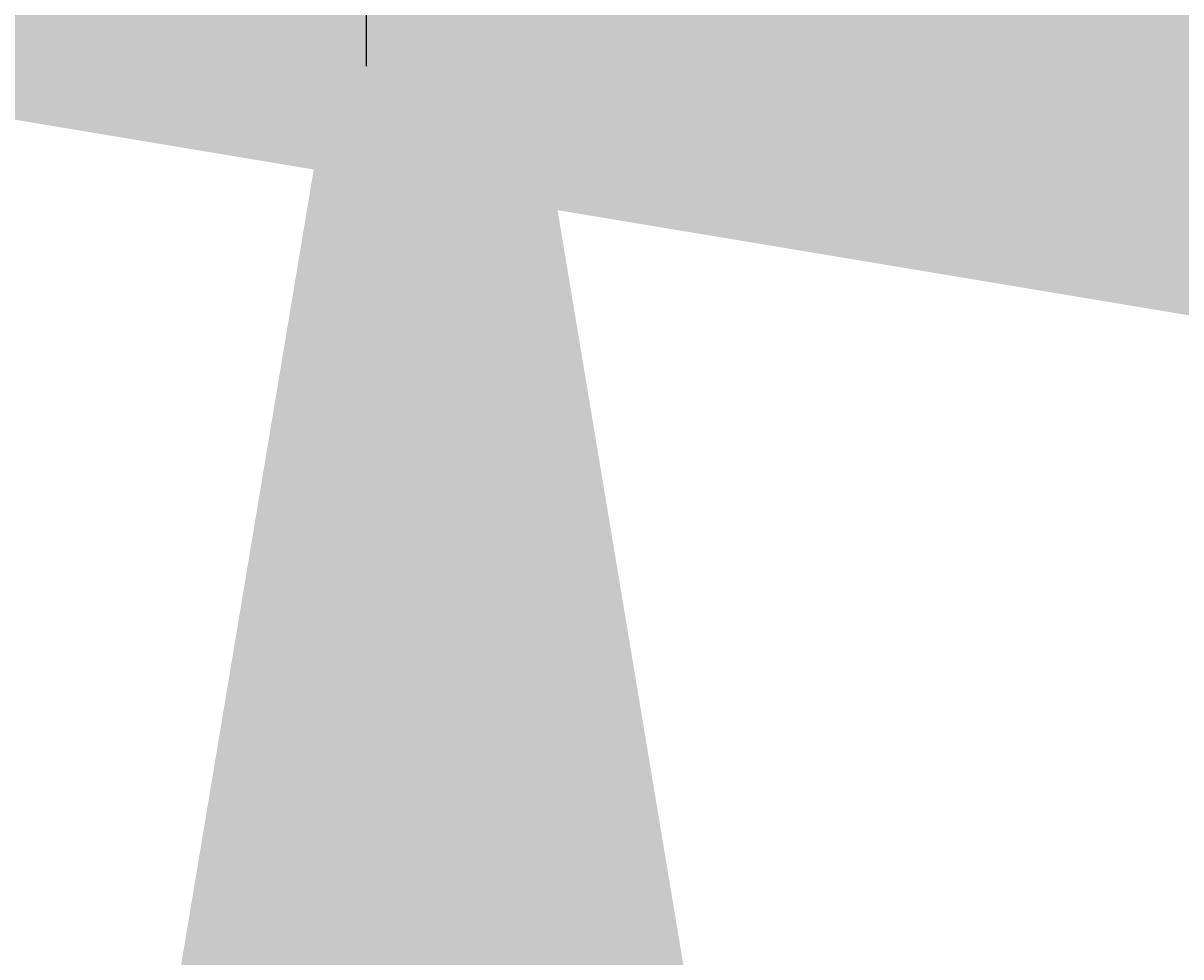
# Model space of a CAD drawing. Units: millimetres. Extents: x -22994 to 29398, y -19990 to 20176.
# Tile 7 of 135: x 211 to 480, y -212 to 5. Entities that reach past the tile are written whole.
import ezdxf

# ---------------------------------------------------------------- set-up
doc = ezdxf.new("R2010")
doc.units = ezdxf.units.MM
doc.header["$MEASUREMENT"] = 0
doc.layers.add('M-DIMS', color=2, linetype='Continuous', lineweight=18)
doc.styles.get("Standard").update_dxf_attribs({"font": 'arial.ttf'})
doc.dimstyles.get("Standard").update_dxf_attribs({"dimtxt": 0.18, "dimasz": 10000, "dimexe": 0.18, "dimexo": 0.0625, "dimgap": 0.09, "dimtad": 0, "dimtih": 1, "dimtoh": 1, "dimdec": 0, "dimzin": 0, "dimdsep": 46, "dimtxsty": 'Standard', "dimcen": 0.09, "dimadec": 0, "dimazin": 0, "dimtfac": 1, "dimtdec": 0, "dimtofl": 0, "dimtmove": 0, "dimatfit": 3, "dimfxl": 1, "dimtolj": 1, "dimtzin": 0, "dimlwd": 30, "dimarcsym": 0})

# ---------------------------------------------------------------- blocks, each defined once
blk = doc.blocks.new('*D2')
at = {"layer": 'Defpoints', "color": 0, "transparency": 16777216}
for p in [(6.68, 10.27), (290.85, 10.27), (290.85, -5.08)]:
    blk.add_point(p, dxfattribs=at)
at = {"layer": 'M-DIMS', "color": 0, "lineweight": -2, "transparency": 16777216}
for p, q in [((6.68, 10.21), (6.68, -5.26)), ((290.85, 10.21), (290.85, -5.26))]:
    blk.add_line(p, q, dxfattribs=at)
at = {"layer": 'M-DIMS', "color": 0, "lineweight": 30, "transparency": 16777216}
for p, q in [((-9993.32, -5.08), (-19993.32, -5.08)), ((10290.85, -5.08), (20290.85, -5.08))]:
    blk.add_line(p, q, dxfattribs=at)
at = {"layer": 'M-DIMS', "color": 0, "transparency": 16777216}
for points in [[(-9993.32, 1661.59), (-9993.32, -1671.75), (6.68, -5.08)], [(10290.85, 1661.59), (10290.85, -1671.75), (290.85, -5.08)]]:
    blk.add_solid(points, dxfattribs=at)
at = {"layer": 'M-DIMS', "color": 0, "transparency": 16777216, "insert": (148.76, -5.08), "char_height": 0.18, "attachment_point": 5}
blk.add_mtext('\\A1;284.2', dxfattribs=at)
blk = doc.blocks.new('*D3')
at = {"layer": 'Defpoints', "color": 0, "transparency": 16777216}
for p in [(110.26, 204.17), (110.26, 176.37), (95.83, 127.97)]:
    blk.add_point(p, dxfattribs=at)
at = {"layer": 'M-DIMS', "color": 0, "lineweight": 30, "transparency": 16777216}
for p, q in [((-9904.17, 204.17), (-19904.17, 204.17)), ((10110.26, 204.17), (20110.26, 204.17))]:
    blk.add_line(p, q, dxfattribs=at)
at = {"layer": 'M-DIMS', "color": 0, "lineweight": -2, "transparency": 16777216}
for p, q in [((95.83, 128.03), (95.83, 204.35)), ((110.26, 176.43), (110.26, 204.35))]:
    blk.add_line(p, q, dxfattribs=at)
at = {"layer": 'M-DIMS', "color": 0, "transparency": 16777216}
for points in [[(-9904.17, 1870.83), (-9904.17, -1462.5), (95.83, 204.17)], [(10110.26, 1870.83), (10110.26, -1462.5), (110.26, 204.17)]]:
    blk.add_solid(points, dxfattribs=at)
at = {"layer": 'M-DIMS', "color": 0, "transparency": 16777216, "insert": (103.05, 204.17), "char_height": 0.18, "attachment_point": 5}
blk.add_mtext('\\A1;14.432', dxfattribs=at)
blk = doc.blocks.new('*D4')
at = {"layer": 'Defpoints', "color": 0, "transparency": 16777216}
for p in [(116.26, 204.17), (110.26, 176.37), (116.26, 176.37)]:
    blk.add_point(p, dxfattribs=at)
at = {"layer": 'M-DIMS', "color": 0, "lineweight": 30, "transparency": 16777216}
for p, q in [((-9889.74, 204.17), (-19889.74, 204.17)), ((10116.26, 204.17), (20116.26, 204.17))]:
    blk.add_line(p, q, dxfattribs=at)
at = {"layer": 'M-DIMS', "color": 0, "lineweight": -2, "transparency": 16777216}
for p, q in [((110.26, 176.43), (110.26, 204.35)), ((116.26, 176.43), (116.26, 204.35))]:
    blk.add_line(p, q, dxfattribs=at)
at = {"layer": 'M-DIMS', "color": 0, "transparency": 16777216}
for points in [[(-9889.74, 1870.83), (-9889.74, -1462.5), (110.26, 204.17)], [(10116.26, 1870.83), (10116.26, -1462.5), (116.26, 204.17)]]:
    blk.add_solid(points, dxfattribs=at)
at = {"layer": 'M-DIMS', "color": 0, "transparency": 16777216, "insert": (113.26, 204.17), "char_height": 0.18, "attachment_point": 5}
blk.add_mtext('\\A1;6', dxfattribs=at)
blk = doc.blocks.new('*D5')
at = {"layer": 'Defpoints', "color": 0, "transparency": 16777216}
for p in [(181.26, 204.17), (116.26, 176.37), (181.26, 176.37)]:
    blk.add_point(p, dxfattribs=at)
at = {"layer": 'M-DIMS', "color": 0, "lineweight": 30, "transparency": 16777216}
for p, q in [((-9883.74, 204.17), (-19883.74, 204.17)), ((10181.26, 204.17), (20181.26, 204.17))]:
    blk.add_line(p, q, dxfattribs=at)
at = {"layer": 'M-DIMS', "color": 0, "lineweight": -2, "transparency": 16777216}
for p, q in [((116.26, 176.43), (116.26, 204.35)), ((181.26, 176.43), (181.26, 204.35))]:
    blk.add_line(p, q, dxfattribs=at)
at = {"layer": 'M-DIMS', "color": 0, "transparency": 16777216}
for points in [[(-9883.74, 1870.83), (-9883.74, -1462.5), (116.26, 204.17)], [(10181.26, 1870.83), (10181.26, -1462.5), (181.26, 204.17)]]:
    blk.add_solid(points, dxfattribs=at)
at = {"layer": 'M-DIMS', "color": 0, "transparency": 16777216, "insert": (148.76, 204.17), "char_height": 0.18, "attachment_point": 5}
blk.add_mtext('\\A1;65', dxfattribs=at)
blk = doc.blocks.new('*D6')
at = {"layer": 'Defpoints', "color": 0, "transparency": 16777216}
for p in [(187.26, 204.17), (181.26, 176.37), (187.26, 176.37)]:
    blk.add_point(p, dxfattribs=at)
at = {"layer": 'M-DIMS', "color": 0, "lineweight": 30, "transparency": 16777216}
for p, q in [((-9818.74, 204.17), (-19818.74, 204.17)), ((10187.26, 204.17), (20187.26, 204.17))]:
    blk.add_line(p, q, dxfattribs=at)
at = {"layer": 'M-DIMS', "color": 0, "lineweight": -2, "transparency": 16777216}
for p, q in [((181.26, 176.43), (181.26, 204.35)), ((187.26, 176.43), (187.26, 204.35))]:
    blk.add_line(p, q, dxfattribs=at)
at = {"layer": 'M-DIMS', "color": 0, "transparency": 16777216}
for points in [[(-9818.74, 1870.83), (-9818.74, -1462.5), (181.26, 204.17)], [(10187.26, 1870.83), (10187.26, -1462.5), (187.26, 204.17)]]:
    blk.add_solid(points, dxfattribs=at)
at = {"layer": 'M-DIMS', "color": 0, "transparency": 16777216, "insert": (184.26, 204.17), "char_height": 0.18, "attachment_point": 5}
blk.add_mtext('\\A1;6', dxfattribs=at)
blk = doc.blocks.new('*D7')
at = {"layer": 'Defpoints', "color": 0, "transparency": 16777216}
for p in [(201.7, 204.17), (187.26, 176.37), (201.7, 127.97)]:
    blk.add_point(p, dxfattribs=at)
at = {"layer": 'M-DIMS', "color": 0, "lineweight": 30, "transparency": 16777216}
for p, q in [((-9812.74, 204.17), (-19812.74, 204.17)), ((10201.7, 204.17), (20201.7, 204.17))]:
    blk.add_line(p, q, dxfattribs=at)
at = {"layer": 'M-DIMS', "color": 0, "lineweight": -2, "transparency": 16777216}
for p, q in [((187.26, 176.43), (187.26, 204.35)), ((201.7, 128.03), (201.7, 204.35))]:
    blk.add_line(p, q, dxfattribs=at)
at = {"layer": 'M-DIMS', "color": 0, "transparency": 16777216}
for points in [[(-9812.74, 1870.83), (-9812.74, -1462.5), (187.26, 204.17)], [(10201.7, 1870.83), (10201.7, -1462.5), (201.7, 204.17)]]:
    blk.add_solid(points, dxfattribs=at)
at = {"layer": 'M-DIMS', "color": 0, "transparency": 16777216, "insert": (194.48, 204.17), "char_height": 0.18, "attachment_point": 5}
blk.add_mtext('\\A1;14.432', dxfattribs=at)
blk = doc.blocks.new('*D8')
at = {"layer": 'Defpoints', "color": 0, "transparency": 16777216}
for p in [(227.65, 204.17), (227.65, 146.73), (201.7, 127.97)]:
    blk.add_point(p, dxfattribs=at)
at = {"layer": 'M-DIMS', "color": 0, "lineweight": 30, "transparency": 16777216}
for p, q in [((-9798.3, 204.17), (-19798.3, 204.17)), ((10227.65, 204.17), (20227.65, 204.17))]:
    blk.add_line(p, q, dxfattribs=at)
at = {"layer": 'M-DIMS', "color": 0, "lineweight": -2, "transparency": 16777216}
for p, q in [((201.7, 128.03), (201.7, 204.35)), ((227.65, 146.79), (227.65, 204.35))]:
    blk.add_line(p, q, dxfattribs=at)
at = {"layer": 'M-DIMS', "color": 0, "transparency": 16777216}
for points in [[(-9798.3, 1870.83), (-9798.3, -1462.5), (201.7, 204.17)], [(10227.65, 1870.83), (10227.65, -1462.5), (227.65, 204.17)]]:
    blk.add_solid(points, dxfattribs=at)
at = {"layer": 'M-DIMS', "color": 0, "transparency": 16777216, "insert": (214.67, 204.17), "char_height": 0.18, "attachment_point": 5}
blk.add_mtext('\\A1;25.95', dxfattribs=at)
blk = doc.blocks.new('*D9')
at = {"layer": 'Defpoints', "color": 0, "transparency": 16777216}
for p in [(187.26, 176.37), (306.2, 176.37), (290.85, 10.27)]:
    blk.add_point(p, dxfattribs=at)
at = {"layer": 'M-DIMS', "color": 0, "lineweight": 30, "transparency": 16777216}
for p, q in [((306.2, 10176.37), (306.2, 20176.37)), ((306.2, -9989.73), (306.2, -19989.73))]:
    blk.add_line(p, q, dxfattribs=at)
at = {"layer": 'M-DIMS', "color": 0, "lineweight": -2, "transparency": 16777216}
for p, q in [((187.33, 176.37), (306.38, 176.37)), ((290.91, 10.27), (306.38, 10.27))]:
    blk.add_line(p, q, dxfattribs=at)
at = {"layer": 'M-DIMS', "color": 0, "transparency": 16777216}
for points in [[(-1360.46, 10176.37), (1972.87, 10176.37), (306.2, 176.37)], [(-1360.46, -9989.73), (1972.87, -9989.73), (306.2, 10.27)]]:
    blk.add_solid(points, dxfattribs=at)
at = {"layer": 'M-DIMS', "color": 0, "transparency": 16777216, "insert": (306.2, 93.32), "char_height": 0.18, "attachment_point": 5}
blk.add_mtext('\\A1;166.1', dxfattribs=at)
blk = doc.blocks.new('*D10')
at = {"layer": 'Defpoints', "color": 0, "transparency": 16777216}
for p in [(125.65, 136.07), (133.35, 136.07), (133.35, -5.08)]:
    blk.add_point(p, dxfattribs=at)
at = {"layer": 'M-DIMS', "color": 0, "lineweight": -2, "transparency": 16777216}
for p, q in [((125.65, 136.01), (125.65, -5.26)), ((133.35, 136.01), (133.35, -5.26))]:
    blk.add_line(p, q, dxfattribs=at)
at = {"layer": 'M-DIMS', "color": 0, "lineweight": 30, "transparency": 16777216}
for p, q in [((-9874.35, -5.08), (-19874.35, -5.08)), ((10133.35, -5.08), (20133.35, -5.08))]:
    blk.add_line(p, q, dxfattribs=at)
at = {"layer": 'M-DIMS', "color": 0, "transparency": 16777216}
for points in [[(-9874.35, 1661.59), (-9874.35, -1671.75), (125.65, -5.08)], [(10133.35, 1661.59), (10133.35, -1671.75), (133.35, -5.08)]]:
    blk.add_solid(points, dxfattribs=at)
at = {"layer": 'M-DIMS', "color": 0, "transparency": 16777216, "insert": (129.5, -5.08), "char_height": 0.18, "attachment_point": 5}
blk.add_mtext('\\A1;7.696', dxfattribs=at)
blk = doc.blocks.new('*D11')
at = {"layer": 'Defpoints', "color": 0, "transparency": 16777216}
for p in [(133.35, 136.07), (135.65, 136.07), (135.65, -5.08)]:
    blk.add_point(p, dxfattribs=at)
at = {"layer": 'M-DIMS', "color": 0, "lineweight": -2, "transparency": 16777216}
for p, q in [((133.35, 136.01), (133.35, -5.26)), ((135.65, 136.01), (135.65, -5.26))]:
    blk.add_line(p, q, dxfattribs=at)
at = {"layer": 'M-DIMS', "color": 0, "lineweight": 30, "transparency": 16777216}
for p, q in [((-9866.65, -5.08), (-19866.65, -5.08)), ((10135.65, -5.08), (20135.65, -5.08))]:
    blk.add_line(p, q, dxfattribs=at)
at = {"layer": 'M-DIMS', "color": 0, "transparency": 16777216}
for points in [[(-9866.65, 1661.59), (-9866.65, -1671.75), (133.35, -5.08)], [(10135.65, 1661.59), (10135.65, -1671.75), (135.65, -5.08)]]:
    blk.add_solid(points, dxfattribs=at)
at = {"layer": 'M-DIMS', "color": 0, "transparency": 16777216, "insert": (134.5, -5.08), "char_height": 0.18, "attachment_point": 5}
blk.add_mtext('\\A1;2.304', dxfattribs=at)
blk = doc.blocks.new('*D12')
at = {"layer": 'Defpoints', "color": 0, "transparency": 16777216}
for p in [(135.65, 136.07), (145.65, 136.07), (145.65, -5.08)]:
    blk.add_point(p, dxfattribs=at)
at = {"layer": 'M-DIMS', "color": 0, "lineweight": -2, "transparency": 16777216}
for p, q in [((135.65, 136.01), (135.65, -5.26)), ((145.65, 136.01), (145.65, -5.26))]:
    blk.add_line(p, q, dxfattribs=at)
at = {"layer": 'M-DIMS', "color": 0, "lineweight": 30, "transparency": 16777216}
for p, q in [((-9864.35, -5.08), (-19864.35, -5.08)), ((10145.65, -5.08), (20145.65, -5.08))]:
    blk.add_line(p, q, dxfattribs=at)
at = {"layer": 'M-DIMS', "color": 0, "transparency": 16777216}
for points in [[(-9864.35, 1661.59), (-9864.35, -1671.75), (135.65, -5.08)], [(10145.65, 1661.59), (10145.65, -1671.75), (145.65, -5.08)]]:
    blk.add_solid(points, dxfattribs=at)
at = {"layer": 'M-DIMS', "color": 0, "transparency": 16777216, "insert": (140.65, -5.08), "char_height": 0.18, "attachment_point": 5}
blk.add_mtext('\\A1;10', dxfattribs=at)
blk = doc.blocks.new('*D13')
at = {"layer": 'Defpoints', "color": 0, "transparency": 16777216}
for p in [(145.65, 136.07), (155.65, 136.07), (155.65, -5.08)]:
    blk.add_point(p, dxfattribs=at)
at = {"layer": 'M-DIMS', "color": 0, "lineweight": -2, "transparency": 16777216}
for p, q in [((145.65, 136.01), (145.65, -5.26)), ((155.65, 136.01), (155.65, -5.26))]:
    blk.add_line(p, q, dxfattribs=at)
at = {"layer": 'M-DIMS', "color": 0, "lineweight": 30, "transparency": 16777216}
for p, q in [((-9854.35, -5.08), (-19854.35, -5.08)), ((10155.65, -5.08), (20155.65, -5.08))]:
    blk.add_line(p, q, dxfattribs=at)
at = {"layer": 'M-DIMS', "color": 0, "transparency": 16777216}
for points in [[(-9854.35, 1661.59), (-9854.35, -1671.75), (145.65, -5.08)], [(10155.65, 1661.59), (10155.65, -1671.75), (155.65, -5.08)]]:
    blk.add_solid(points, dxfattribs=at)
at = {"layer": 'M-DIMS', "color": 0, "transparency": 16777216, "insert": (150.65, -5.08), "char_height": 0.18, "attachment_point": 5}
blk.add_mtext('\\A1;10', dxfattribs=at)
blk = doc.blocks.new('*D14')
at = {"layer": 'Defpoints', "color": 0, "transparency": 16777216}
for p in [(155.65, 136.07), (165.65, 136.07), (165.65, -5.08)]:
    blk.add_point(p, dxfattribs=at)
at = {"layer": 'M-DIMS', "color": 0, "lineweight": -2, "transparency": 16777216}
for p, q in [((155.65, 136.01), (155.65, -5.26)), ((165.65, 136.01), (165.65, -5.26))]:
    blk.add_line(p, q, dxfattribs=at)
at = {"layer": 'M-DIMS', "color": 0, "lineweight": 30, "transparency": 16777216}
for p, q in [((-9844.35, -5.08), (-19844.35, -5.08)), ((10165.65, -5.08), (20165.65, -5.08))]:
    blk.add_line(p, q, dxfattribs=at)
at = {"layer": 'M-DIMS', "color": 0, "transparency": 16777216}
for points in [[(-9844.35, 1661.59), (-9844.35, -1671.75), (155.65, -5.08)], [(10165.65, 1661.59), (10165.65, -1671.75), (165.65, -5.08)]]:
    blk.add_solid(points, dxfattribs=at)
at = {"layer": 'M-DIMS', "color": 0, "transparency": 16777216, "insert": (160.65, -5.08), "char_height": 0.18, "attachment_point": 5}
blk.add_mtext('\\A1;10', dxfattribs=at)
blk = doc.blocks.new('*D15')
at = {"layer": 'Defpoints', "color": 0, "transparency": 16777216}
for p in [(173.35, 154.79), (173.35, 136.07), (306.2, 136.07)]:
    blk.add_point(p, dxfattribs=at)
at = {"layer": 'M-DIMS', "color": 0, "lineweight": 30, "transparency": 16777216}
for p, q in [((306.2, 10154.79), (306.2, 20154.79)), ((306.2, -9863.93), (306.2, -19863.93))]:
    blk.add_line(p, q, dxfattribs=at)
at = {"layer": 'M-DIMS', "color": 0, "lineweight": -2, "transparency": 16777216}
for p, q in [((173.41, 154.79), (306.38, 154.79)), ((173.41, 136.07), (306.38, 136.07))]:
    blk.add_line(p, q, dxfattribs=at)
at = {"layer": 'M-DIMS', "color": 0, "transparency": 16777216}
for points in [[(-1360.46, 10154.79), (1972.87, 10154.79), (306.2, 154.79)], [(-1360.46, -9863.93), (1972.87, -9863.93), (306.2, 136.07)]]:
    blk.add_solid(points, dxfattribs=at)
at = {"layer": 'M-DIMS', "color": 0, "transparency": 16777216, "insert": (306.2, 145.43), "char_height": 0.18, "attachment_point": 5}
blk.add_mtext('\\A1;18.717', dxfattribs=at)
blk = doc.blocks.new('*D16')
at = {"layer": 'Defpoints', "color": 0, "transparency": 16777216}
for p in [(120.17, 204.17), (110.47, 48.03), (120.17, 48.03)]:
    blk.add_point(p, dxfattribs=at)
at = {"layer": 'M-DIMS', "color": 0, "lineweight": 30, "transparency": 16777216}
for p, q in [((-9889.53, 204.17), (-19889.53, 204.17)), ((10120.17, 204.17), (20120.17, 204.17))]:
    blk.add_line(p, q, dxfattribs=at)
at = {"layer": 'M-DIMS', "color": 0, "lineweight": -2, "transparency": 16777216}
for p, q in [((110.47, 48.1), (110.47, 204.35)), ((120.17, 48.1), (120.17, 204.35))]:
    blk.add_line(p, q, dxfattribs=at)
at = {"layer": 'M-DIMS', "color": 0, "transparency": 16777216}
for points in [[(-9889.53, 1870.83), (-9889.53, -1462.5), (110.47, 204.17)], [(10120.17, 1870.83), (10120.17, -1462.5), (120.17, 204.17)]]:
    blk.add_solid(points, dxfattribs=at)
at = {"layer": 'M-DIMS', "color": 0, "transparency": 16777216, "insert": (115.32, 204.17), "char_height": 0.18, "attachment_point": 5}
blk.add_mtext('\\A1;9.704', dxfattribs=at)
blk = doc.blocks.new('*D17')
at = {"layer": 'Defpoints', "color": 0, "transparency": 16777216}
for p in [(126.17, 204.17), (120.17, 48.03), (126.17, 48.03)]:
    blk.add_point(p, dxfattribs=at)
at = {"layer": 'M-DIMS', "color": 0, "lineweight": 30, "transparency": 16777216}
for p, q in [((-9879.83, 204.17), (-19879.83, 204.17)), ((10126.17, 204.17), (20126.17, 204.17))]:
    blk.add_line(p, q, dxfattribs=at)
at = {"layer": 'M-DIMS', "color": 0, "lineweight": -2, "transparency": 16777216}
for p, q in [((120.17, 48.1), (120.17, 204.35)), ((126.17, 48.1), (126.17, 204.35))]:
    blk.add_line(p, q, dxfattribs=at)
at = {"layer": 'M-DIMS', "color": 0, "transparency": 16777216}
for points in [[(-9879.83, 1870.83), (-9879.83, -1462.5), (120.17, 204.17)], [(10126.17, 1870.83), (10126.17, -1462.5), (126.17, 204.17)]]:
    blk.add_solid(points, dxfattribs=at)
at = {"layer": 'M-DIMS', "color": 0, "transparency": 16777216, "insert": (123.17, 204.17), "char_height": 0.18, "attachment_point": 5}
blk.add_mtext('\\A1;6', dxfattribs=at)
blk = doc.blocks.new('*D18')
at = {"layer": 'Defpoints', "color": 0, "transparency": 16777216}
for p in [(132.17, 204.17), (126.17, 48.03), (132.17, 48.03)]:
    blk.add_point(p, dxfattribs=at)
at = {"layer": 'M-DIMS', "color": 0, "lineweight": 30, "transparency": 16777216}
for p, q in [((-9873.83, 204.17), (-19873.83, 204.17)), ((10132.17, 204.17), (20132.17, 204.17))]:
    blk.add_line(p, q, dxfattribs=at)
at = {"layer": 'M-DIMS', "color": 0, "lineweight": -2, "transparency": 16777216}
for p, q in [((126.17, 48.1), (126.17, 204.35)), ((132.17, 48.1), (132.17, 204.35))]:
    blk.add_line(p, q, dxfattribs=at)
at = {"layer": 'M-DIMS', "color": 0, "transparency": 16777216}
for points in [[(-9873.83, 1870.83), (-9873.83, -1462.5), (126.17, 204.17)], [(10132.17, 1870.83), (10132.17, -1462.5), (132.17, 204.17)]]:
    blk.add_solid(points, dxfattribs=at)
at = {"layer": 'M-DIMS', "color": 0, "transparency": 16777216, "insert": (129.17, 204.17), "char_height": 0.18, "attachment_point": 5}
blk.add_mtext('\\A1;6', dxfattribs=at)
blk = doc.blocks.new('*D19')
at = {"layer": 'Defpoints', "color": 0, "transparency": 16777216}
for p in [(138.17, 204.17), (132.17, 48.03), (138.17, 48.03)]:
    blk.add_point(p, dxfattribs=at)
at = {"layer": 'M-DIMS', "color": 0, "lineweight": 30, "transparency": 16777216}
for p, q in [((-9867.83, 204.17), (-19867.83, 204.17)), ((10138.17, 204.17), (20138.17, 204.17))]:
    blk.add_line(p, q, dxfattribs=at)
at = {"layer": 'M-DIMS', "color": 0, "lineweight": -2, "transparency": 16777216}
for p, q in [((132.17, 48.1), (132.17, 204.35)), ((138.17, 48.1), (138.17, 204.35))]:
    blk.add_line(p, q, dxfattribs=at)
at = {"layer": 'M-DIMS', "color": 0, "transparency": 16777216}
for points in [[(-9867.83, 1870.83), (-9867.83, -1462.5), (132.17, 204.17)], [(10138.17, 1870.83), (10138.17, -1462.5), (138.17, 204.17)]]:
    blk.add_solid(points, dxfattribs=at)
at = {"layer": 'M-DIMS', "color": 0, "transparency": 16777216, "insert": (135.17, 204.17), "char_height": 0.18, "attachment_point": 5}
blk.add_mtext('\\A1;6', dxfattribs=at)
blk = doc.blocks.new('*D20')
at = {"layer": 'Defpoints', "color": 0, "transparency": 16777216}
for p in [(144.17, 204.17), (138.17, 48.03), (144.17, 48.03)]:
    blk.add_point(p, dxfattribs=at)
at = {"layer": 'M-DIMS', "color": 0, "lineweight": 30, "transparency": 16777216}
for p, q in [((-9861.83, 204.17), (-19861.83, 204.17)), ((10144.17, 204.17), (20144.17, 204.17))]:
    blk.add_line(p, q, dxfattribs=at)
at = {"layer": 'M-DIMS', "color": 0, "lineweight": -2, "transparency": 16777216}
for p, q in [((138.17, 48.1), (138.17, 204.35)), ((144.17, 48.1), (144.17, 204.35))]:
    blk.add_line(p, q, dxfattribs=at)
at = {"layer": 'M-DIMS', "color": 0, "transparency": 16777216}
for points in [[(-9861.83, 1870.83), (-9861.83, -1462.5), (138.17, 204.17)], [(10144.17, 1870.83), (10144.17, -1462.5), (144.17, 204.17)]]:
    blk.add_solid(points, dxfattribs=at)
at = {"layer": 'M-DIMS', "color": 0, "transparency": 16777216, "insert": (141.17, 204.17), "char_height": 0.18, "attachment_point": 5}
blk.add_mtext('\\A1;6', dxfattribs=at)
blk = doc.blocks.new('*D21')
at = {"layer": 'Defpoints', "color": 0, "transparency": 16777216}
for p in [(149.12, 204.17), (144.17, 48.03), (149.12, 48.03)]:
    blk.add_point(p, dxfattribs=at)
at = {"layer": 'M-DIMS', "color": 0, "lineweight": 30, "transparency": 16777216}
for p, q in [((-9855.83, 204.17), (-19855.83, 204.17)), ((10149.12, 204.17), (20149.12, 204.17))]:
    blk.add_line(p, q, dxfattribs=at)
at = {"layer": 'M-DIMS', "color": 0, "lineweight": -2, "transparency": 16777216}
for p, q in [((144.17, 48.1), (144.17, 204.35)), ((149.12, 48.1), (149.12, 204.35))]:
    blk.add_line(p, q, dxfattribs=at)
at = {"layer": 'M-DIMS', "color": 0, "transparency": 16777216}
for points in [[(-9855.83, 1870.83), (-9855.83, -1462.5), (144.17, 204.17)], [(10149.12, 1870.83), (10149.12, -1462.5), (149.12, 204.17)]]:
    blk.add_solid(points, dxfattribs=at)
at = {"layer": 'M-DIMS', "color": 0, "transparency": 16777216, "insert": (146.64, 204.17), "char_height": 0.18, "attachment_point": 5}
blk.add_mtext('\\A1;4.945', dxfattribs=at)
blk = doc.blocks.new('*D22')
at = {"layer": 'Defpoints', "color": 0, "transparency": 16777216}
for p in [(149.12, 30.99), (155.12, 30.99), (155.12, -5.08)]:
    blk.add_point(p, dxfattribs=at)
at = {"layer": 'M-DIMS', "color": 0, "lineweight": -2, "transparency": 16777216}
for p, q in [((149.12, 30.93), (149.12, -5.26)), ((155.12, 30.93), (155.12, -5.26))]:
    blk.add_line(p, q, dxfattribs=at)
at = {"layer": 'M-DIMS', "color": 0, "lineweight": 30, "transparency": 16777216}
for p, q in [((-9850.88, -5.08), (-19850.88, -5.08)), ((10155.12, -5.08), (20155.12, -5.08))]:
    blk.add_line(p, q, dxfattribs=at)
at = {"layer": 'M-DIMS', "color": 0, "transparency": 16777216}
for points in [[(-9850.88, 1661.59), (-9850.88, -1671.75), (149.12, -5.08)], [(10155.12, 1661.59), (10155.12, -1671.75), (155.12, -5.08)]]:
    blk.add_solid(points, dxfattribs=at)
at = {"layer": 'M-DIMS', "color": 0, "transparency": 16777216, "insert": (152.12, -5.08), "char_height": 0.18, "attachment_point": 5}
blk.add_mtext('\\A1;6', dxfattribs=at)
blk = doc.blocks.new('*D23')
at = {"layer": 'Defpoints', "color": 0, "transparency": 16777216}
for p in [(155.12, 30.99), (161.12, 30.99), (161.12, -5.08)]:
    blk.add_point(p, dxfattribs=at)
at = {"layer": 'M-DIMS', "color": 0, "lineweight": -2, "transparency": 16777216}
for p, q in [((155.12, 30.93), (155.12, -5.26)), ((161.12, 30.93), (161.12, -5.26))]:
    blk.add_line(p, q, dxfattribs=at)
at = {"layer": 'M-DIMS', "color": 0, "lineweight": 30, "transparency": 16777216}
for p, q in [((-9844.88, -5.08), (-19844.88, -5.08)), ((10161.12, -5.08), (20161.12, -5.08))]:
    blk.add_line(p, q, dxfattribs=at)
at = {"layer": 'M-DIMS', "color": 0, "transparency": 16777216}
for points in [[(-9844.88, 1661.59), (-9844.88, -1671.75), (155.12, -5.08)], [(10161.12, 1661.59), (10161.12, -1671.75), (161.12, -5.08)]]:
    blk.add_solid(points, dxfattribs=at)
at = {"layer": 'M-DIMS', "color": 0, "transparency": 16777216, "insert": (158.12, -5.08), "char_height": 0.18, "attachment_point": 5}
blk.add_mtext('\\A1;6', dxfattribs=at)
blk = doc.blocks.new('*D24')
at = {"layer": 'Defpoints', "color": 0, "transparency": 16777216}
for p in [(161.12, 30.99), (166.44, 30.99), (166.44, -5.08)]:
    blk.add_point(p, dxfattribs=at)
at = {"layer": 'M-DIMS', "color": 0, "lineweight": -2, "transparency": 16777216}
for p, q in [((161.12, 30.93), (161.12, -5.26)), ((166.44, 30.93), (166.44, -5.26))]:
    blk.add_line(p, q, dxfattribs=at)
at = {"layer": 'M-DIMS', "color": 0, "lineweight": 30, "transparency": 16777216}
for p, q in [((-9838.88, -5.08), (-19838.88, -5.08)), ((10166.44, -5.08), (20166.44, -5.08))]:
    blk.add_line(p, q, dxfattribs=at)
at = {"layer": 'M-DIMS', "color": 0, "transparency": 16777216}
for points in [[(-9838.88, 1661.59), (-9838.88, -1671.75), (161.12, -5.08)], [(10166.44, 1661.59), (10166.44, -1671.75), (166.44, -5.08)]]:
    blk.add_solid(points, dxfattribs=at)
at = {"layer": 'M-DIMS', "color": 0, "transparency": 16777216, "insert": (163.78, -5.08), "char_height": 0.18, "attachment_point": 5}
blk.add_mtext('\\A1;5.323', dxfattribs=at)
blk = doc.blocks.new('*D25')
at = {"layer": 'Defpoints', "color": 0, "transparency": 16777216}
for p in [(166.44, 30.99), (172.44, 30.99), (172.44, -5.08)]:
    blk.add_point(p, dxfattribs=at)
at = {"layer": 'M-DIMS', "color": 0, "lineweight": -2, "transparency": 16777216}
for p, q in [((166.44, 30.93), (166.44, -5.26)), ((172.44, 30.93), (172.44, -5.26))]:
    blk.add_line(p, q, dxfattribs=at)
at = {"layer": 'M-DIMS', "color": 0, "lineweight": 30, "transparency": 16777216}
for p, q in [((-9833.56, -5.08), (-19833.56, -5.08)), ((10172.44, -5.08), (20172.44, -5.08))]:
    blk.add_line(p, q, dxfattribs=at)
at = {"layer": 'M-DIMS', "color": 0, "transparency": 16777216}
for points in [[(-9833.56, 1661.59), (-9833.56, -1671.75), (166.44, -5.08)], [(10172.44, 1661.59), (10172.44, -1671.75), (172.44, -5.08)]]:
    blk.add_solid(points, dxfattribs=at)
at = {"layer": 'M-DIMS', "color": 0, "transparency": 16777216, "insert": (169.44, -5.08), "char_height": 0.18, "attachment_point": 5}
blk.add_mtext('\\A1;6', dxfattribs=at)
blk = doc.blocks.new('*D26')
at = {"layer": 'Defpoints', "color": 0, "transparency": 16777216}
for p in [(172.44, 30.99), (178.44, 30.99), (178.44, -5.08)]:
    blk.add_point(p, dxfattribs=at)
at = {"layer": 'M-DIMS', "color": 0, "lineweight": -2, "transparency": 16777216}
for p, q in [((172.44, 30.93), (172.44, -5.26)), ((178.44, 30.93), (178.44, -5.26))]:
    blk.add_line(p, q, dxfattribs=at)
at = {"layer": 'M-DIMS', "color": 0, "lineweight": 30, "transparency": 16777216}
for p, q in [((-9827.56, -5.08), (-19827.56, -5.08)), ((10178.44, -5.08), (20178.44, -5.08))]:
    blk.add_line(p, q, dxfattribs=at)
at = {"layer": 'M-DIMS', "color": 0, "transparency": 16777216}
for points in [[(-9827.56, 1661.59), (-9827.56, -1671.75), (172.44, -5.08)], [(10178.44, 1661.59), (10178.44, -1671.75), (178.44, -5.08)]]:
    blk.add_solid(points, dxfattribs=at)
at = {"layer": 'M-DIMS', "color": 0, "transparency": 16777216, "insert": (175.44, -5.08), "char_height": 0.18, "attachment_point": 5}
blk.add_mtext('\\A1;6', dxfattribs=at)
blk = doc.blocks.new('*D27')
at = {"layer": 'Defpoints', "color": 0, "transparency": 16777216}
for p in [(178.44, 30.99), (188.12, 30.99), (188.12, -5.08)]:
    blk.add_point(p, dxfattribs=at)
at = {"layer": 'M-DIMS', "color": 0, "lineweight": -2, "transparency": 16777216}
for p, q in [((178.44, 30.93), (178.44, -5.26)), ((188.12, 30.93), (188.12, -5.26))]:
    blk.add_line(p, q, dxfattribs=at)
at = {"layer": 'M-DIMS', "color": 0, "lineweight": 30, "transparency": 16777216}
for p, q in [((-9821.56, -5.08), (-19821.56, -5.08)), ((10188.12, -5.08), (20188.12, -5.08))]:
    blk.add_line(p, q, dxfattribs=at)
at = {"layer": 'M-DIMS', "color": 0, "transparency": 16777216}
for points in [[(-9821.56, 1661.59), (-9821.56, -1671.75), (178.44, -5.08)], [(10188.12, 1661.59), (10188.12, -1671.75), (188.12, -5.08)]]:
    blk.add_solid(points, dxfattribs=at)
at = {"layer": 'M-DIMS', "color": 0, "transparency": 16777216, "insert": (183.28, -5.08), "char_height": 0.18, "attachment_point": 5}
blk.add_mtext('\\A1;9.679', dxfattribs=at)
blk = doc.blocks.new('*D28')
at = {"layer": 'Defpoints', "color": 0, "transparency": 16777216}
for p in [(188.12, 48.03), (306.2, 48.03), (188.12, 30.99)]:
    blk.add_point(p, dxfattribs=at)
at = {"layer": 'M-DIMS', "color": 0, "lineweight": 30, "transparency": 16777216}
for p, q in [((306.2, 10048.03), (306.2, 20048.03)), ((306.2, -9969.01), (306.2, -19969.01))]:
    blk.add_line(p, q, dxfattribs=at)
at = {"layer": 'M-DIMS', "color": 0, "lineweight": -2, "transparency": 16777216}
for p, q in [((188.18, 48.03), (306.38, 48.03)), ((188.18, 30.99), (306.38, 30.99))]:
    blk.add_line(p, q, dxfattribs=at)
at = {"layer": 'M-DIMS', "color": 0, "transparency": 16777216}
for points in [[(-1360.46, 10048.03), (1972.87, 10048.03), (306.2, 48.03)], [(-1360.46, -9969.01), (1972.87, -9969.01), (306.2, 30.99)]]:
    blk.add_solid(points, dxfattribs=at)
at = {"layer": 'M-DIMS', "color": 0, "transparency": 16777216, "insert": (306.2, 39.51), "char_height": 0.18, "attachment_point": 5}
blk.add_mtext('\\A1;17.045', dxfattribs=at)
blk = doc.blocks.new('*D29')
at = {"layer": 'Defpoints', "color": 0, "transparency": 16777216}
for p in [(36.8, 80.04), (64.03, 80.04)]:
    blk.add_point(p, dxfattribs=at)
at = {"layer": 'M-DIMS', "color": 0, "lineweight": -2, "transparency": 16777216}
for p, q in [((50.33, 80.04), (50.51, 80.04)), ((50.42, 79.96), (50.42, 80.14))]:
    blk.add_line(p, q, dxfattribs=at)
at = {"layer": 'M-DIMS', "color": 0, "lineweight": 30, "transparency": 16777216}
blk.add_line((20064.03, 80.03), (10064.03, 80.04), dxfattribs=at)
at = {"layer": 'M-DIMS', "color": 0, "transparency": 16777216}
blk.add_solid([(10064.03, 1746.7), (10064.03, -1586.63), (64.03, 80.04)], dxfattribs=at)
at = {"layer": 'M-DIMS', "color": 0, "transparency": 16777216, "insert": (20064.52, 80.03), "char_height": 0.18, "attachment_point": 5}
blk.add_mtext('\\A1;∅27.23', dxfattribs=at)
blk = doc.blocks.new('*D30')
at = {"layer": 'Defpoints', "color": 0, "transparency": 16777216}
for p in [(216.31, 146.73), (238.98, 146.73)]:
    blk.add_point(p, dxfattribs=at)
at = {"layer": 'M-DIMS', "color": 0, "lineweight": -2, "transparency": 16777216}
for p, q in [((227.56, 146.73), (227.74, 146.73)), ((227.65, 146.64), (227.65, 146.82))]:
    blk.add_line(p, q, dxfattribs=at)
at = {"layer": 'M-DIMS', "color": 0, "lineweight": 30, "transparency": 16777216}
blk.add_line((20238.98, 147.5), (10238.98, 147.11), dxfattribs=at)
at = {"layer": 'M-DIMS', "color": 0, "transparency": 16777216}
blk.add_solid([(10238.92, 1813.78), (10239.05, -1519.55), (238.98, 146.73)], dxfattribs=at)
at = {"layer": 'M-DIMS', "color": 0, "transparency": 16777216, "insert": (20239.54, 147.5), "char_height": 0.18, "attachment_point": 5}
blk.add_mtext('\\A1;∅22.667', dxfattribs=at)
blk = doc.blocks.new('*D31')
at = {"layer": 'Defpoints', "color": 0, "transparency": 16777216}
for p in [(223.16, 146.73), (232.13, 146.73)]:
    blk.add_point(p, dxfattribs=at)
at = {"layer": 'M-DIMS', "color": 0, "lineweight": 30, "transparency": 16777216}
blk.add_line((20232.13, 148.67), (10232.13, 147.7), dxfattribs=at)
at = {"layer": 'M-DIMS', "color": 0, "lineweight": -2, "transparency": 16777216}
for p, q in [((227.56, 146.73), (227.74, 146.73)), ((227.65, 146.64), (227.65, 146.82))]:
    blk.add_line(p, q, dxfattribs=at)
at = {"layer": 'M-DIMS', "color": 0, "transparency": 16777216}
blk.add_solid([(10231.97, 1814.36), (10232.29, -1518.97), (232.13, 146.73)], dxfattribs=at)
at = {"layer": 'M-DIMS', "color": 0, "transparency": 16777216, "insert": (20232.62, 148.67), "char_height": 0.18, "attachment_point": 5}
blk.add_mtext('\\A1;∅8.969', dxfattribs=at)
blk = doc.blocks.new('*D33')
at = {"layer": 'Defpoints', "color": 0, "transparency": 16777216}
for p in [(229.56, 154.38), (233, 153.35)]:
    blk.add_point(p, dxfattribs=at)
at = {"layer": 'M-DIMS', "color": 0, "lineweight": -2, "transparency": 16777216}
for p, q in [((229.47, 154.38), (229.65, 154.38)), ((229.56, 154.29), (229.56, 154.47))]:
    blk.add_line(p, q, dxfattribs=at)
at = {"layer": 'M-DIMS', "color": 0, "lineweight": 30, "transparency": 16777216}
for p, q in [((19396.34, -5570.84), (9814.67, -2708.74)), ((29396.34, -5570.84), (19396.34, -5570.84))]:
    blk.add_line(p, q, dxfattribs=at)
at = {"layer": 'M-DIMS', "color": 0, "transparency": 16777216}
blk.add_solid([(10291.68, -1111.8), (9337.65, -4305.69), (233, 153.35)], dxfattribs=at)
at = {"layer": 'M-DIMS', "color": 0, "transparency": 16777216, "insert": (29397.01, -5570.84), "char_height": 0.18, "attachment_point": 5}
blk.add_mtext('\\A1;6X R3.586', dxfattribs=at)
blk = doc.blocks.new('*D37')
at = {"layer": 'Defpoints', "color": 0, "transparency": 16777216}
for p in [(54.83, 118.61), (59.49, 118.61)]:
    blk.add_point(p, dxfattribs=at)
at = {"layer": 'M-DIMS', "color": 0, "lineweight": -2, "transparency": 16777216}
for p, q in [((57.07, 118.61), (57.25, 118.61)), ((57.16, 118.52), (57.16, 118.7))]:
    blk.add_line(p, q, dxfattribs=at)
at = {"layer": 'M-DIMS', "color": 0, "lineweight": 30, "transparency": 16777216}
blk.add_line((20059.49, 116.25), (10059.49, 117.43), dxfattribs=at)
at = {"layer": 'M-DIMS', "color": 0, "transparency": 16777216}
blk.add_solid([(10059.69, 1784.1), (10059.3, -1549.23), (59.49, 118.61)], dxfattribs=at)
at = {"layer": 'M-DIMS', "color": 0, "transparency": 16777216, "insert": (20059.99, 116.25), "char_height": 0.18, "attachment_point": 5}
blk.add_mtext('\\A1;∅4.659', dxfattribs=at)

msp = doc.modelspace()

# ---------------------------------------------------------------- dimensions: what is measured, and where the dimension line sits
at = {"layer": 'M-DIMS'}
for base, p1, p2, override, picture, middle in [((306.202, 176.3662), (290.852, 10.2713), (187.2647, 176.3662), {"dimdec": 1, "dimlfac": 1, "dimrnd": 0, "dimzin": 0, "dimdsep": 46, "dimlunit": 2}, '*D9', (306.202, 93.3187)), ((306.202, 136.0713), (173.3459, 154.788), (173.3459, 136.0713), {"dimdec": 3, "dimlfac": 1, "dimrnd": 0, "dimzin": 0, "dimdsep": 46, "dimlunit": 2}, '*D15', (306.202, 145.4297)), ((306.202, 48.0349), (188.1175, 30.9895), (188.1175, 48.0349), {"dimdec": 3, "dimlfac": 1, "dimrnd": 0, "dimzin": 0, "dimdsep": 46, "dimlunit": 2}, '*D28', (306.202, 39.5122))]:
    dim = msp.add_linear_dim(base=base, p1=p1, p2=p2, angle=90, dimstyle='Standard', override=override, dxfattribs=at)
    dim.commit()
    dim.dimension.update_dxf_attribs({"geometry": picture, "text_midpoint": middle})
for base, p1, p2, override, picture, middle in [((110.2647, 204.1654), (95.8327, 127.967), (110.2647, 176.3662), {"dimdec": 3, "dimlfac": 1, "dimrnd": 0, "dimzin": 0, "dimdsep": 46, "dimlunit": 2}, '*D3', (103.0487, 204.1654)), ((116.2647, 204.1654), (110.2647, 176.3662), (116.2647, 176.3662), {"dimdec": 0, "dimlfac": 1, "dimrnd": 0, "dimzin": 0, "dimdsep": 46, "dimlunit": 2}, '*D4', (113.2647, 204.1654)), ((120.1702, 204.1654), (110.4658, 48.0349), (120.1702, 48.0349), {"dimdec": 3, "dimlfac": 1, "dimrnd": 0, "dimzin": 0, "dimdsep": 46, "dimlunit": 2}, '*D16', (115.318, 204.1654)), ((181.2647, 204.1654), (116.2647, 176.3662), (181.2647, 176.3662), {"dimdec": 0, "dimlfac": 1, "dimrnd": 0, "dimzin": 0, "dimdsep": 46, "dimlunit": 2}, '*D5', (148.7647, 204.1654)), ((126.1702, 204.1654), (120.1702, 48.0349), (126.1702, 48.0349), {"dimdec": 0, "dimlfac": 1, "dimrnd": 0, "dimzin": 0, "dimdsep": 46, "dimlunit": 2}, '*D17', (123.1702, 204.1654)), ((132.1702, 204.1654), (126.1702, 48.0349), (132.1702, 48.0349), {"dimdec": 0, "dimlfac": 1, "dimrnd": 0, "dimzin": 0, "dimdsep": 46, "dimlunit": 2}, '*D18', (129.1702, 204.1654)), ((138.1702, 204.1654), (132.1702, 48.0349), (138.1702, 48.0349), {"dimdec": 0, "dimlfac": 1, "dimrnd": 0, "dimzin": 0, "dimdsep": 46, "dimlunit": 2}, '*D19', (135.1702, 204.1654)), ((144.1702, 204.1654), (138.1702, 48.0349), (144.1702, 48.0349), {"dimdec": 0, "dimlfac": 1, "dimrnd": 0, "dimzin": 0, "dimdsep": 46, "dimlunit": 2}, '*D20', (141.1702, 204.1654)), ((149.11567, 204.16539), (144.17023, 48.03494), (149.11567, 48.03494), {"dimdec": 3, "dimlfac": 1, "dimrnd": 0, "dimzin": 0, "dimdsep": 46, "dimlunit": 2}, '*D21', (146.64295, 204.16539)), ((187.2647, 204.1654), (181.2647, 176.3662), (187.2647, 176.3662), {"dimdec": 0, "dimlfac": 1, "dimrnd": 0, "dimzin": 0, "dimdsep": 46, "dimlunit": 2}, '*D6', (184.2647, 204.1654)), ((201.6967, 204.1654), (187.2647, 176.3662), (201.6967, 127.967), {"dimdec": 3, "dimlfac": 1, "dimrnd": 0, "dimzin": 0, "dimdsep": 46, "dimlunit": 2}, '*D7', (194.4807, 204.1654)), ((227.6485, 204.1654), (201.6967, 127.967), (227.6485, 146.7296), {"dimdec": 2, "dimlfac": 1, "dimrnd": 0, "dimzin": 0, "dimdsep": 46, "dimlunit": 2}, '*D8', (214.6726, 204.1654)), ((290.852, -5.0787), (6.6773, 10.2713), (290.852, 10.2713), {"dimdec": 1, "dimlfac": 1, "dimrnd": 0, "dimzin": 0, "dimdsep": 46, "dimlunit": 2}, '*D2', (148.7647, -5.0787)), ((133.3459, -5.0787), (125.6498, 136.0713), (133.3459, 136.0713), {"dimdec": 3, "dimlfac": 1, "dimrnd": 0, "dimzin": 0, "dimdsep": 46, "dimlunit": 2}, '*D10', (129.4978, -5.0787)), ((135.6498, -5.0787), (133.3459, 136.0713), (135.6498, 136.0713), {"dimdec": 3, "dimlfac": 1, "dimrnd": 0, "dimzin": 0, "dimdsep": 46, "dimlunit": 2}, '*D11', (134.4978, -5.0787)), ((145.6498, -5.0787), (135.6498, 136.0713), (145.6498, 136.0713), {"dimdec": 0, "dimlfac": 1, "dimrnd": 0, "dimzin": 0, "dimdsep": 46, "dimlunit": 2}, '*D12', (140.6498, -5.0787)), ((155.6498, -5.0787), (145.6498, 136.0713), (155.6498, 136.0713), {"dimdec": 0, "dimlfac": 1, "dimrnd": 0, "dimzin": 0, "dimdsep": 46, "dimlunit": 2}, '*D13', (150.6498, -5.0787)), ((155.1157, -5.0787), (149.1157, 30.9895), (155.1157, 30.9895), {"dimdec": 0, "dimlfac": 1, "dimrnd": 0, "dimzin": 0, "dimdsep": 46, "dimlunit": 2}, '*D22', (152.1157, -5.0787)), ((161.1157, -5.0787), (155.1157, 30.9895), (161.1157, 30.9895), {"dimdec": 0, "dimlfac": 1, "dimrnd": 0, "dimzin": 0, "dimdsep": 46, "dimlunit": 2}, '*D23', (158.1157, -5.0787)), ((165.6498, -5.0787), (155.6498, 136.0713), (165.6498, 136.0713), {"dimdec": 0, "dimlfac": 1, "dimrnd": 0, "dimzin": 0, "dimdsep": 46, "dimlunit": 2}, '*D14', (160.6498, -5.0787)), ((166.4387, -5.0787), (161.1157, 30.9895), (166.4387, 30.9895), {"dimdec": 3, "dimlfac": 1, "dimrnd": 0, "dimzin": 0, "dimdsep": 46, "dimlunit": 2}, '*D24', (163.7772, -5.0787)), ((172.4387, -5.0787), (166.4387, 30.9895), (172.4387, 30.9895), {"dimdec": 0, "dimlfac": 1, "dimrnd": 0, "dimzin": 0, "dimdsep": 46, "dimlunit": 2}, '*D25', (169.4387, -5.0787)), ((178.4387, -5.0787), (172.4387, 30.9895), (178.4387, 30.9895), {"dimdec": 0, "dimlfac": 1, "dimrnd": 0, "dimzin": 0, "dimdsep": 46, "dimlunit": 2}, '*D26', (175.4387, -5.0787)), ((188.1175, -5.0787), (178.4387, 30.9895), (188.1175, 30.9895), {"dimdec": 3, "dimlfac": 1, "dimrnd": 0, "dimzin": 0, "dimdsep": 46, "dimlunit": 2}, '*D27', (183.2781, -5.0787))]:
    dim = msp.add_linear_dim(base=base, p1=p1, p2=p2, dimstyle='Standard', override=override, dxfattribs=at)
    dim.commit()
    dim.dimension.update_dxf_attribs({"geometry": picture, "text_midpoint": middle})
for p1, p2, picture, middle in [((223.1641, 146.7291), (232.1328, 146.73), '*D31', (20232.1327, 148.6656)), ((216.3148, 146.7291), (238.9821, 146.73), '*D30', (20238.9821, 147.4959))]:
    dim = msp.add_diameter_dim_2p(p1=p1, p2=p2, dimstyle='Standard', override={"dimdec": 3, "dimlfac": 1, "dimrnd": 0, "dimzin": 0, "dimdsep": 46, "dimlunit": 2}, dxfattribs=at)
    dim.commit()
    dim.dimension.update_dxf_attribs({"geometry": picture, "text_midpoint": middle, "dimtype": 163})
for p1, p2, override, picture, middle in [((54.8343, 118.6145), (59.4936, 118.614), {"dimdec": 3, "dimlfac": 1, "dimrnd": 0, "dimzin": 0, "dimdsep": 46, "dimlunit": 2}, '*D37', (20059.4934, 116.2531)), ((36.8006, 80.045), (64.0296, 80.045), {"dimdec": 2, "dimlfac": 1, "dimrnd": 0, "dimzin": 0, "dimdsep": 46, "dimlunit": 2}, '*D29', (20064.0296, 80.0303))]:
    dim = msp.add_diameter_dim_2p(p1=p1, p2=p2, dimstyle='Standard', override=override, dxfattribs=at)
    dim.commit()
    dim.dimension.update_dxf_attribs({"geometry": picture, "text_midpoint": middle})
dim = msp.add_radius_dim(center=(229.5613, 154.3773), mpoint=(232.9972, 153.3509), text='6X <>', dimstyle='Standard', override={"dimdec": 3, "dimlfac": 1, "dimrnd": 0, "dimzin": 0, "dimdsep": 46, "dimlunit": 2}, dxfattribs=at)
dim.commit()
dim.dimension.update_dxf_attribs({"geometry": '*D33', "text_midpoint": (29397.0125, -5570.8378)})

doc.saveas('drawing.dxf')
